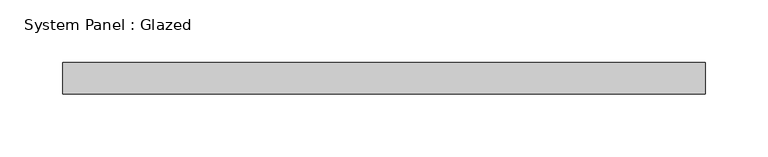
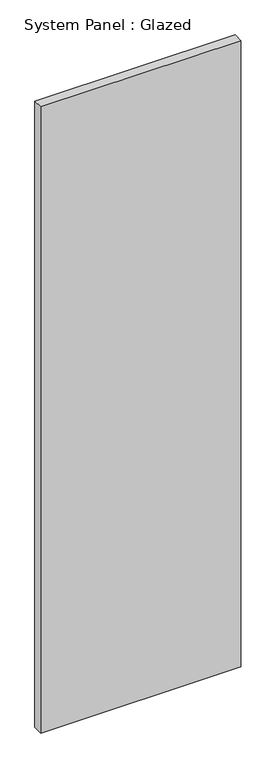
"""IFC4 building model written with IfcOpenShell, lengths in millimetres: plate geometry, System Panel : Glazed."""

from ifc_helpers import new_model, si_unit, origin, origin_with_axes, place, context, project, spatial, polyline, outline, extrude, source, transform, mapped, element, save


def system_panel_glazed_078fe0dd(model_context):
    return source(origin(), model_context, "Body", "SweptSolid", [
        extrude(outline(polyline([(257.175, 19.05), (-257.175, 19.05), (-257.175, 44.45), (257.175, 44.45), (257.175, 19.05)])), origin_with_axes(), (0.0, 0.0, 1.0), 1701.8),
    ])


if __name__ == "__main__":
    model = new_model("IFC4")
    model_context = context("Model", 3, world=origin())
    ifc_project = project(units=[si_unit("LENGTHUNIT", "METRE", prefix="MILLI")], contexts=[model_context])
    site = spatial("IfcSite", under=ifc_project)
    building = spatial("IfcBuilding", under=site)
    placement = place(None, origin())
    system_panel_glazed_shape = system_panel_glazed_078fe0dd(model_context)
    element("IfcPlate", 1, ObjectType="System Panel : Glazed", at=placement, inside=building, context=model_context, shape_type="MappedRepresentation", body=[
        mapped(system_panel_glazed_shape, transform((0.0, 0.0, 0.0), x_axis=(1.0, 0.0, 0.0), y_axis=(0.0, 1.0, 0.0), z_axis=(0.0, 0.0, 1.0))),
    ])
    save(model, "model.ifc")

# Revit data of these elements
# Type "System Panel : Glazed"
#   Construction Type Id = "GSP4R"
#   Analytic Construction = "1/8 in Pilkington single glazing"
#   Visual Light Transmittance = 0.9
#   Solar Heat Gain Coefficient = 0.86
#   Heat Transfer Coefficient (U) = 1.18115 BTU/(h·ft²·°F)
#   Define Thermal Properties by = 1
# Element 1 (IfcPlate, "System Panel : Glazed")
#   Materials on its faces: "Glass"
# Materials
#   "Glass": class "Glass", colour RGB 0 128 192, transparency 0.75, Description = "Soda Lime Glass", Cost = 0
